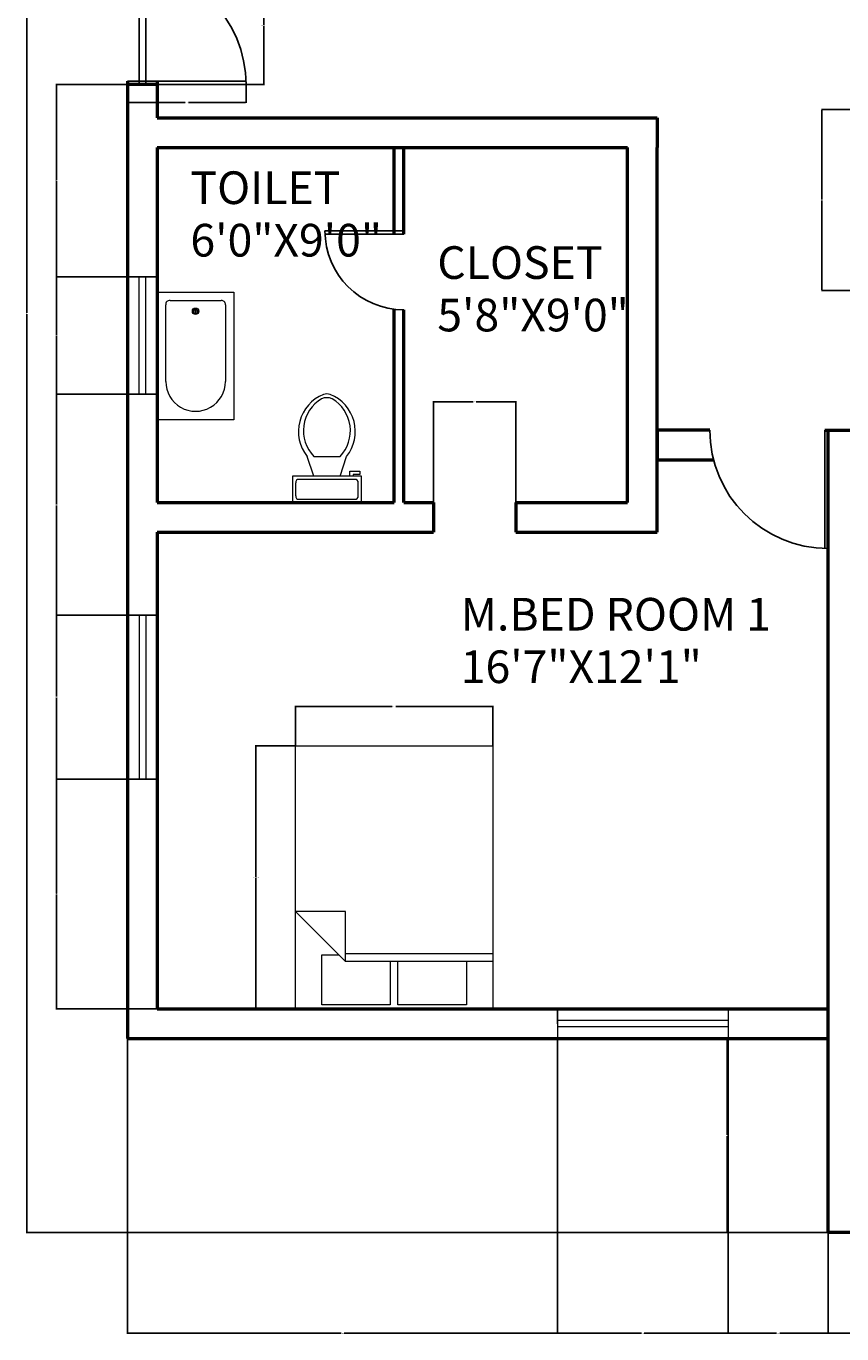
# Model space of a CAD drawing. Units: inches. Extents: x 614 to 1202, y 131 to 752.
# Tile 1 of 5: x 614 to 862, y 131 to 529. Entities that reach past the tile are written whole.
import ezdxf

# ---------------------------------------------------------------- set-up
doc = ezdxf.new("R2010")
doc.units = ezdxf.units.IN
doc.header["$MEASUREMENT"] = 0
for name, color, linetype, lineweight in [('A-ANNO-DIMS', 2, 'Continuous', 18), ('A-AREA-IDEN', 7, 'Continuous', 18), ('A-DOOR', 3, 'Continuous', 25), ('A-FLOR-FIXT', 9, 'Continuous', 18), ('A-FURN', 8, 'Continuous', 18), ('A-GLAZ', 4, 'Continuous', 18), ('A-WALL', 7, 'Continuous', 50)]:
    doc.layers.add(name, color=color, linetype=linetype, lineweight=lineweight)
doc.styles.get("Standard").update_dxf_attribs({"font": 'arial.ttf'})
doc.dimstyles.get("Standard").update_dxf_attribs({"dimtxt": 0.18, "dimasz": 0.18, "dimexe": 0.18, "dimexo": 0.0625, "dimgap": 0.09, "dimtad": 0, "dimtih": 1, "dimtoh": 1, "dimdec": 0, "dimzin": 0, "dimdsep": 46, "dimlunit": 3, "dimtxsty": 'Standard', "dimcen": 0.09, "dimadec": 0, "dimazin": 0, "dimtfac": 1, "dimtdec": 0, "dimtofl": 0, "dimtmove": 0, "dimatfit": 3, "dimfxl": 1, "dimtolj": 1, "dimtzin": 0, "dimarcsym": 0})

# ---------------------------------------------------------------- blocks, each defined once
blk = doc.blocks.new('Bed - Queen')
for p, q in [((0, -80.00003), (0, 0)), ((0, 0), (59.99999, 0)), ((59.99999, 0), (59.99999, -80.00003)), ((7.99999, -1.2), (28.79998, -1.2)), ((7.99999, -14.4), (7.99999, -1.2)), ((28.79998, -1.2), (28.79998, -14.4)), ((31.19999, -1.2), (51.99999, -1.2)), ((31.19999, -14.4), (31.19999, -1.2)), ((51.99999, -1.2), (51.99999, -16.4)), ((0, -14.4), (44.8, -14.4)), ((59.99999, -29.6), (44.8, -14.4)), ((44.8, -14.4), (44.8, -29.6)), ((44.8, -16.8), (0, -16.8)), ((51.99999, -16.4), (46.79936, -16.4)), ((44.8, -29.6), (59.99999, -29.6)), ((59.99999, -80.00003), (0, -80.00003))]:
    blk.add_line(p, q)
blk = doc.blocks.new('Toilet - top')
for p, q in [((9.5, -6), (9.5, -2)), ((-10, -8.5), (-8, -8.5)), ((-10, -9.5), (-10, -8.5)), ((-7, -9.5), (-10, -9.5)), ((-8, -8.5), (-8, -8)), ((-7, -8), (-7, -9.5)), ((-4, -8), (-6, -14)), ((4, -8), (6, -14)), ((4, -14), (-4, -14))]:
    blk.add_line(p, q)
blk.add_lwpolyline([(10.5, -8), (10.5, 0), (-10.5, 0), (-10.5, -8)], close=True)
for points in [[(-9.5, -2), (-9.5, -6)], [(8.5, -1), (-8.5, -1)], [(-8.5, -7), (8.5, -7)]]:
    blk.add_lwpolyline(points)
for centre, radius, start, end in [((-8.62, -1.88), 0.884, 81.8699, 188.1301), ((8.62, -1.88), 0.884, 351.8699, 98.1301), ((-8.62, -6.12), 0.884, 171.8699, 278.1301), ((8.62, -6.12), 0.884, 261.8699, 8.1301), ((3.52, -21.58), 12.17, 141.4691, 247.9714), ((4.2, -21.82), 11.33, 136.3677, 238.9468), ((-3.52, -21.58), 12.17, 292.0284, 38.5307), ((-4.2, -21.82), 11.33, 301.053, 43.6321), ((0, -27.88), 4, 245.7318, 294.2682), ((0, -29), 4, 254.8605, 285.1395)]:
    blk.add_arc(centre, radius, start, end)
blk = doc.blocks.new('Bath Tub - 26 x 60 in.')
for p, q in [((8, -18), (10, -18)), ((9, -17), (9, -19))]:
    blk.add_line(p, q)
blk.add_lwpolyline([(0, -36), (0, 0), (60, 0), (60, -36)], close=True)
for points in [[(4, -30), (4, -6)], [(6, -4), (42, -4)], [(42, -32), (6, -32)]]:
    blk.add_lwpolyline(points)
for radius in [1.5, 1]:
    blk.add_circle((9, -18), radius)
for centre, radius, start, end in [((5.75, -5.75), 1.77, 81.8699, 188.1301), ((42, -18), 14, 270, 90), ((5.75, -30.25), 1.77, 171.8699, 278.1301)]:
    blk.add_arc(centre, radius, start, end)
blk = doc.blocks.new('DOOR-SINGLE-36IN')
for p, q in [((0, 1), (36, 1)), ((0, 0), (36, 0))]:
    blk.add_line(p, q)
blk.add_arc((0, 0), 36, 0, 90)
blk = doc.blocks.new('DOOR-SINGLE-24IN')
for p, q in [((0, 0), (0, 24)), ((1, 0), (1, 24))]:
    blk.add_line(p, q)
blk.add_arc((0, 0), 24, 0, 90)
blk = doc.blocks.new('*D15')
at = {"layer": 'A-ANNO-DIMS', "color": 0, "lineweight": -2, "transparency": 16777216}
for p, q in [((681.06, 547.36), (686.57, 547.36)), ((686.39, 547.18), (686.39, 529.54)), ((686.39, 511.54), (686.39, 529.18)), ((681.06, 511.36), (686.57, 511.36))]:
    blk.add_line(p, q, dxfattribs=at)
at = {"layer": 'A-ANNO-DIMS', "color": 0, "transparency": 16777216}
for points in [[(686.36, 547.18), (686.42, 547.18), (686.39, 547.36)], [(686.36, 511.54), (686.42, 511.54), (686.39, 511.36)]]:
    blk.add_solid(points, dxfattribs=at)
at = {"layer": 'Defpoints', "color": 0, "transparency": 16777216}
for p in [(680.99, 547.36), (686.39, 547.36), (680.99, 511.36)]:
    blk.add_point(p, dxfattribs=at)
at = {"layer": 'A-ANNO-DIMS', "color": 0, "transparency": 16777216, "insert": (686.39, 529.36), "char_height": 0.18, "attachment_point": 5}
blk.add_mtext('\\A1;DOOR 36 TYP.', dxfattribs=at)
blk = doc.blocks.new('*D16')
at = {"layer": 'A-ANNO-DIMS', "color": 0, "lineweight": -2, "transparency": 16777216}
for p, q in [((644.99, 511.3), (644.99, 505.78)), ((680.99, 511.3), (680.99, 505.78)), ((645.17, 505.96), (662.47, 505.96)), ((680.81, 505.96), (663.52, 505.96))]:
    blk.add_line(p, q, dxfattribs=at)
at = {"layer": 'A-ANNO-DIMS', "color": 0, "transparency": 16777216}
for points in [[(645.17, 505.99), (645.17, 505.93), (644.99, 505.96)], [(680.81, 505.99), (680.81, 505.93), (680.99, 505.96)]]:
    blk.add_solid(points, dxfattribs=at)
at = {"layer": 'Defpoints', "color": 0, "transparency": 16777216}
for p in [(644.99, 511.36), (680.99, 511.36), (680.99, 505.96)]:
    blk.add_point(p, dxfattribs=at)
at = {"layer": 'A-ANNO-DIMS', "color": 0, "transparency": 16777216, "insert": (662.99, 505.96), "char_height": 0.18, "attachment_point": 5}
blk.add_mtext('\\A1;36 TYP.', dxfattribs=at)
blk = doc.blocks.new('*D23')
at = {"layer": 'A-ANNO-DIMS', "color": 0, "lineweight": -2, "transparency": 16777216}
for p, q in [((695.93, 310.26), (683.81, 310.26)), ((683.99, 310.08), (683.99, 270.45)), ((683.99, 230.44), (683.99, 270.08)), ((695.93, 230.26), (683.81, 230.26))]:
    blk.add_line(p, q, dxfattribs=at)
at = {"layer": 'A-ANNO-DIMS', "color": 0, "transparency": 16777216}
for points in [[(683.96, 310.08), (684.02, 310.08), (683.99, 310.26)], [(683.96, 230.44), (684.02, 230.44), (683.99, 230.26)]]:
    blk.add_solid(points, dxfattribs=at)
at = {"layer": 'Defpoints', "color": 0, "transparency": 16777216}
for p in [(695.99, 310.26), (683.99, 230.26), (695.99, 230.26)]:
    blk.add_point(p, dxfattribs=at)
at = {"layer": 'A-ANNO-DIMS', "color": 0, "transparency": 16777216, "insert": (683.99, 270.26), "char_height": 0.18, "attachment_point": 5}
blk.add_mtext('\\A1;QUEEN BED 80 TYP.', dxfattribs=at)
blk = doc.blocks.new('*D24')
at = {"layer": 'A-ANNO-DIMS', "color": 0, "lineweight": -2, "transparency": 16777216}
for p, q in [((695.99, 310.33), (695.99, 322.44)), ((696.17, 322.26), (725.47, 322.26)), ((755.81, 322.26), (726.52, 322.26)), ((755.99, 310.33), (755.99, 322.44))]:
    blk.add_line(p, q, dxfattribs=at)
at = {"layer": 'A-ANNO-DIMS', "color": 0, "transparency": 16777216}
for points in [[(696.17, 322.29), (696.17, 322.23), (695.99, 322.26)], [(755.81, 322.29), (755.81, 322.23), (755.99, 322.26)]]:
    blk.add_solid(points, dxfattribs=at)
at = {"layer": 'Defpoints', "color": 0, "transparency": 16777216}
for p in [(695.99, 322.26), (695.99, 310.26), (755.99, 310.26)]:
    blk.add_point(p, dxfattribs=at)
at = {"layer": 'A-ANNO-DIMS', "color": 0, "transparency": 16777216, "insert": (725.99, 322.26), "char_height": 0.18, "attachment_point": 5}
blk.add_mtext('\\A1;60 TYP.', dxfattribs=at)
blk = doc.blocks.new('*D34')
at = {"layer": 'A-ANNO-DIMS', "color": 0, "lineweight": -2, "transparency": 16777216}
for p, q in [((869.71, 503.76), (855.94, 503.76)), ((856.12, 503.58), (856.12, 476.44)), ((856.12, 448.94), (856.12, 476.08)), ((869.71, 448.76), (855.94, 448.76))]:
    blk.add_line(p, q, dxfattribs=at)
at = {"layer": 'A-ANNO-DIMS', "color": 0, "transparency": 16777216}
for points in [[(856.09, 503.58), (856.15, 503.58), (856.12, 503.76)], [(856.09, 448.94), (856.15, 448.94), (856.12, 448.76)]]:
    blk.add_solid(points, dxfattribs=at)
at = {"layer": 'Defpoints', "color": 0, "transparency": 16777216}
for p in [(856.12, 503.76), (869.77, 503.76), (869.77, 448.76)]:
    blk.add_point(p, dxfattribs=at)
at = {"layer": 'A-ANNO-DIMS', "color": 0, "transparency": 16777216, "insert": (856.12, 476.26), "char_height": 0.18, "attachment_point": 5}
blk.add_mtext('\\A1;55', dxfattribs=at)
blk = doc.blocks.new('*D36')
at = {"layer": 'A-ANNO-DIMS', "color": 0, "lineweight": -2, "transparency": 16777216}
for p, q in [((644.93, 721.26), (614.16, 721.26)), ((614.34, 721.08), (614.34, 441.95)), ((614.34, 162.44), (614.34, 441.58)), ((857.93, 162.26), (614.16, 162.26))]:
    blk.add_line(p, q, dxfattribs=at)
at = {"layer": 'A-ANNO-DIMS', "color": 0, "transparency": 16777216}
for points in [[(614.31, 721.08), (614.37, 721.08), (614.34, 721.26)], [(614.31, 162.44), (614.37, 162.44), (614.34, 162.26)]]:
    blk.add_solid(points, dxfattribs=at)
at = {"layer": 'Defpoints', "color": 0, "transparency": 16777216}
for p in [(614.34, 721.26), (644.99, 721.26), (857.99, 162.26)]:
    blk.add_point(p, dxfattribs=at)
at = {"layer": 'A-ANNO-DIMS', "color": 0, "transparency": 16777216, "insert": (614.34, 441.76), "char_height": 0.18, "attachment_point": 5}
blk.add_mtext('\\A1;559', dxfattribs=at)
blk = doc.blocks.new('*D47')
at = {"layer": 'A-ANNO-DIMS', "color": 0, "lineweight": -2, "transparency": 16777216}
for p, q in [((653.93, 511.36), (623.16, 511.36)), ((623.34, 511.18), (623.34, 482.33)), ((623.34, 453.11), (623.34, 481.96)), ((653.93, 452.93), (623.16, 452.93))]:
    blk.add_line(p, q, dxfattribs=at)
at = {"layer": 'A-ANNO-DIMS', "color": 0, "transparency": 16777216}
for points in [[(623.31, 511.18), (623.37, 511.18), (623.34, 511.36)], [(623.31, 453.11), (623.37, 453.11), (623.34, 452.93)]]:
    blk.add_solid(points, dxfattribs=at)
at = {"layer": 'Defpoints', "color": 0, "transparency": 16777216}
for p in [(623.34, 511.36), (653.99, 511.36), (653.99, 452.93)]:
    blk.add_point(p, dxfattribs=at)
at = {"layer": 'A-ANNO-DIMS', "color": 0, "transparency": 16777216, "insert": (623.34, 482.15), "char_height": 0.18, "attachment_point": 5}
blk.add_mtext('\\A1;58.42', dxfattribs=at)
blk = doc.blocks.new('*D48')
at = {"layer": 'A-ANNO-DIMS', "color": 0, "lineweight": -2, "transparency": 16777216}
for p, q in [((653.93, 452.93), (623.16, 452.93)), ((623.34, 452.75), (623.34, 435.26)), ((623.34, 417.4), (623.34, 434.9)), ((653.93, 417.22), (623.16, 417.22))]:
    blk.add_line(p, q, dxfattribs=at)
at = {"layer": 'A-ANNO-DIMS', "color": 0, "transparency": 16777216}
for points in [[(623.31, 452.75), (623.37, 452.75), (623.34, 452.93)], [(623.31, 417.4), (623.37, 417.4), (623.34, 417.22)]]:
    blk.add_solid(points, dxfattribs=at)
at = {"layer": 'Defpoints', "color": 0, "transparency": 16777216}
for p in [(623.34, 452.93), (653.99, 452.93), (653.99, 417.22)]:
    blk.add_point(p, dxfattribs=at)
at = {"layer": 'A-ANNO-DIMS', "color": 0, "transparency": 16777216, "insert": (623.34, 435.08), "char_height": 0.18, "attachment_point": 5}
blk.add_mtext('\\A1;35.71', dxfattribs=at)
blk = doc.blocks.new('*D49')
at = {"layer": 'A-ANNO-DIMS', "color": 0, "lineweight": -2, "transparency": 16777216}
for p, q in [((653.93, 417.22), (623.16, 417.22)), ((623.34, 417.04), (623.34, 383.77)), ((623.34, 350.13), (623.34, 383.4)), ((653.93, 349.95), (623.16, 349.95))]:
    blk.add_line(p, q, dxfattribs=at)
at = {"layer": 'A-ANNO-DIMS', "color": 0, "transparency": 16777216}
for points in [[(623.31, 417.04), (623.37, 417.04), (623.34, 417.22)], [(623.31, 350.13), (623.37, 350.13), (623.34, 349.95)]]:
    blk.add_solid(points, dxfattribs=at)
at = {"layer": 'Defpoints', "color": 0, "transparency": 16777216}
for p in [(623.34, 417.22), (653.99, 417.22), (653.99, 349.95)]:
    blk.add_point(p, dxfattribs=at)
at = {"layer": 'A-ANNO-DIMS', "color": 0, "transparency": 16777216, "insert": (623.34, 383.58), "char_height": 0.18, "attachment_point": 5}
blk.add_mtext('\\A1;67.28', dxfattribs=at)
blk = doc.blocks.new('*D50')
at = {"layer": 'A-ANNO-DIMS', "color": 0, "lineweight": -2, "transparency": 16777216}
for p, q in [((653.93, 349.95), (623.16, 349.95)), ((623.34, 349.77), (623.34, 325.24)), ((623.34, 300.35), (623.34, 324.87)), ((653.93, 300.17), (623.16, 300.17))]:
    blk.add_line(p, q, dxfattribs=at)
at = {"layer": 'A-ANNO-DIMS', "color": 0, "transparency": 16777216}
for points in [[(623.31, 349.77), (623.37, 349.77), (623.34, 349.95)], [(623.31, 300.35), (623.37, 300.35), (623.34, 300.17)]]:
    blk.add_solid(points, dxfattribs=at)
at = {"layer": 'Defpoints', "color": 0, "transparency": 16777216}
for p in [(623.34, 349.95), (653.99, 349.95), (653.99, 300.17)]:
    blk.add_point(p, dxfattribs=at)
at = {"layer": 'A-ANNO-DIMS', "color": 0, "transparency": 16777216, "insert": (623.34, 325.06), "char_height": 0.18, "attachment_point": 5}
blk.add_mtext('\\A1;49.78', dxfattribs=at)
blk = doc.blocks.new('*D51')
at = {"layer": 'A-ANNO-DIMS', "color": 0, "lineweight": -2, "transparency": 16777216}
for p, q in [((653.93, 300.17), (623.16, 300.17)), ((623.34, 299.99), (623.34, 265.4)), ((623.34, 230.44), (623.34, 265.03)), ((653.93, 230.26), (623.16, 230.26))]:
    blk.add_line(p, q, dxfattribs=at)
at = {"layer": 'A-ANNO-DIMS', "color": 0, "transparency": 16777216}
for points in [[(623.31, 299.99), (623.37, 299.99), (623.34, 300.17)], [(623.31, 230.44), (623.37, 230.44), (623.34, 230.26)]]:
    blk.add_solid(points, dxfattribs=at)
at = {"layer": 'Defpoints', "color": 0, "transparency": 16777216}
for p in [(623.34, 300.17), (653.99, 300.17), (653.99, 230.26)]:
    blk.add_point(p, dxfattribs=at)
at = {"layer": 'A-ANNO-DIMS', "color": 0, "transparency": 16777216, "insert": (623.34, 265.21), "char_height": 0.18, "attachment_point": 5}
blk.add_mtext('\\A1;69.9', dxfattribs=at)
blk = doc.blocks.new('*D61')
at = {"layer": 'A-ANNO-DIMS', "color": 0, "lineweight": -2, "transparency": 16777216}
for p, q in [((644.99, 221.2), (644.99, 131.43)), ((775.74, 221.2), (775.74, 131.43)), ((645.17, 131.61), (709.91, 131.61)), ((775.56, 131.61), (710.82, 131.61))]:
    blk.add_line(p, q, dxfattribs=at)
at = {"layer": 'A-ANNO-DIMS', "color": 0, "transparency": 16777216}
for points in [[(645.17, 131.64), (645.17, 131.58), (644.99, 131.61)], [(775.56, 131.64), (775.56, 131.58), (775.74, 131.61)]]:
    blk.add_solid(points, dxfattribs=at)
at = {"layer": 'Defpoints', "color": 0, "transparency": 16777216}
for p in [(644.99, 221.26), (775.74, 221.26), (775.74, 131.61)]:
    blk.add_point(p, dxfattribs=at)
at = {"layer": 'A-ANNO-DIMS', "color": 0, "transparency": 16777216, "insert": (710.37, 131.61), "char_height": 0.18, "attachment_point": 5}
blk.add_mtext('\\A1;130.75', dxfattribs=at)
blk = doc.blocks.new('*D62')
at = {"layer": 'A-ANNO-DIMS', "color": 0, "lineweight": -2, "transparency": 16777216}
for p, q in [((775.74, 221.2), (775.74, 131.43)), ((827.61, 221.2), (827.61, 131.43)), ((775.92, 131.61), (801.28, 131.61)), ((827.43, 131.61), (802.07, 131.61))]:
    blk.add_line(p, q, dxfattribs=at)
at = {"layer": 'A-ANNO-DIMS', "color": 0, "transparency": 16777216}
for points in [[(775.92, 131.64), (775.92, 131.58), (775.74, 131.61)], [(827.43, 131.64), (827.43, 131.58), (827.61, 131.61)]]:
    blk.add_solid(points, dxfattribs=at)
at = {"layer": 'Defpoints', "color": 0, "transparency": 16777216}
for p in [(775.74, 221.26), (827.61, 221.26), (827.61, 131.61)]:
    blk.add_point(p, dxfattribs=at)
at = {"layer": 'A-ANNO-DIMS', "color": 0, "transparency": 16777216, "insert": (801.68, 131.61), "char_height": 0.18, "attachment_point": 5}
blk.add_mtext('\\A1;51.86', dxfattribs=at)
blk = doc.blocks.new('*D63')
at = {"layer": 'A-ANNO-DIMS', "color": 0, "lineweight": -2, "transparency": 16777216}
for p, q in [((827.61, 221.2), (827.61, 131.43)), ((857.99, 162.2), (857.99, 131.43)), ((827.79, 131.61), (842.34, 131.61)), ((857.81, 131.61), (843.26, 131.61))]:
    blk.add_line(p, q, dxfattribs=at)
at = {"layer": 'A-ANNO-DIMS', "color": 0, "transparency": 16777216}
for points in [[(827.79, 131.64), (827.79, 131.58), (827.61, 131.61)], [(857.81, 131.64), (857.81, 131.58), (857.99, 131.61)]]:
    blk.add_solid(points, dxfattribs=at)
at = {"layer": 'Defpoints', "color": 0, "transparency": 16777216}
for p in [(827.61, 221.26), (857.99, 162.26), (857.99, 131.61)]:
    blk.add_point(p, dxfattribs=at)
at = {"layer": 'A-ANNO-DIMS', "color": 0, "transparency": 16777216, "insert": (842.8, 131.61), "char_height": 0.18, "attachment_point": 5}
blk.add_mtext('\\A1;30.386', dxfattribs=at)
blk = doc.blocks.new('*D64')
at = {"layer": 'A-ANNO-DIMS', "color": 0, "lineweight": -2, "transparency": 16777216}
for p, q in [((857.99, 162.2), (857.99, 131.43)), ((1016.99, 162.2), (1016.99, 131.43)), ((858.17, 131.61), (937.21, 131.61)), ((1016.81, 131.61), (937.77, 131.61))]:
    blk.add_line(p, q, dxfattribs=at)
at = {"layer": 'A-ANNO-DIMS', "color": 0, "transparency": 16777216}
for points in [[(858.17, 131.64), (858.17, 131.58), (857.99, 131.61)], [(1016.81, 131.64), (1016.81, 131.58), (1016.99, 131.61)]]:
    blk.add_solid(points, dxfattribs=at)
at = {"layer": 'Defpoints', "color": 0, "transparency": 16777216}
for p in [(857.99, 162.26), (1016.99, 162.26), (1016.99, 131.61)]:
    blk.add_point(p, dxfattribs=at)
at = {"layer": 'A-ANNO-DIMS', "color": 0, "transparency": 16777216, "insert": (937.49, 131.61), "char_height": 0.18, "attachment_point": 5}
blk.add_mtext('\\A1;159', dxfattribs=at)
blk = doc.blocks.new('*D68')
at = {"layer": 'A-ANNO-DIMS', "color": 0, "lineweight": -2, "transparency": 16777216}
for p, q in [((857.93, 221.26), (827.16, 221.26)), ((827.34, 221.08), (827.34, 191.95)), ((827.34, 162.44), (827.34, 191.58)), ((857.93, 162.26), (827.16, 162.26))]:
    blk.add_line(p, q, dxfattribs=at)
at = {"layer": 'A-ANNO-DIMS', "color": 0, "transparency": 16777216}
for points in [[(827.31, 221.08), (827.37, 221.08), (827.34, 221.26)], [(827.31, 162.44), (827.37, 162.44), (827.34, 162.26)]]:
    blk.add_solid(points, dxfattribs=at)
at = {"layer": 'Defpoints', "color": 0, "transparency": 16777216}
for p in [(827.34, 221.26), (857.99, 221.26), (857.99, 162.26)]:
    blk.add_point(p, dxfattribs=at)
at = {"layer": 'A-ANNO-DIMS', "color": 0, "transparency": 16777216, "insert": (827.34, 191.76), "char_height": 0.18, "attachment_point": 5}
blk.add_mtext('\\A1;59', dxfattribs=at)
blk = doc.blocks.new('*D79')
at = {"layer": 'A-ANNO-DIMS', "color": 0, "lineweight": -2, "transparency": 16777216}
for p, q in [((737.99, 384.33), (737.99, 415.09)), ((738.17, 414.91), (750.03, 414.91)), ((762.81, 414.91), (750.96, 414.91)), ((762.99, 384.33), (762.99, 415.09))]:
    blk.add_line(p, q, dxfattribs=at)
at = {"layer": 'A-ANNO-DIMS', "color": 0, "transparency": 16777216}
for points in [[(738.17, 414.94), (738.17, 414.88), (737.99, 414.91)], [(762.81, 414.94), (762.81, 414.88), (762.99, 414.91)]]:
    blk.add_solid(points, dxfattribs=at)
at = {"layer": 'Defpoints', "color": 0, "transparency": 16777216}
for p in [(762.99, 414.91), (737.99, 384.26), (762.99, 384.26)]:
    blk.add_point(p, dxfattribs=at)
at = {"layer": 'A-ANNO-DIMS', "color": 0, "transparency": 16777216, "insert": (750.49, 414.91), "char_height": 0.18, "attachment_point": 5}
blk.add_mtext('\\A1;25.006', dxfattribs=at)

msp = doc.modelspace()

# ---------------------------------------------------------------- linework, layer by layer
at = {"layer": 'A-DOOR'}
for p, q in [((648.4938, 511.3589), (648.4938, 547.1883)), ((650.4938, 511.3589), (650.4938, 546.9362)), ((644.9938, 511.3589), (644.9938, 512.3589)), ((728.9938, 466.8602), (728.9938, 465.8602))]:
    msp.add_line(p, q, dxfattribs=at)
at = {"layer": 'A-GLAZ'}
for p, q in [((653.9938, 452.934), (644.9938, 452.934)), ((648.4938, 417.2227), (648.4938, 452.934)), ((649.4938, 452.934), (653.9938, 452.934)), ((650.4938, 417.2227), (650.4938, 452.934)), ((653.9938, 417.2227), (644.9938, 417.2227)), ((653.9938, 349.9459), (644.9938, 349.9459)), ((648.4938, 349.9459), (648.4938, 300.1655)), ((650.4938, 349.9459), (650.4938, 300.1655)), ((653.9938, 300.1655), (644.9938, 300.1655)), ((649.4938, 300.1655), (653.9938, 300.1655)), ((775.7442, 225.7636), (775.7442, 230.2636)), ((775.7442, 230.2636), (775.7442, 221.2636)), ((827.6082, 226.7636), (775.7442, 226.7636)), ((827.6082, 230.2636), (827.6082, 221.2636)), ((827.6082, 224.7636), (775.7442, 224.7636))]:
    msp.add_line(p, q, dxfattribs=at)
at = {"layer": 'A-WALL'}
for p, q in [((644.9938, 512.3589), (644.9938, 221.2636)), ((653.9938, 511.3589), (644.9938, 511.3589)), ((653.9938, 512.3589), (653.9938, 501.2636)), ((653.9938, 501.2636), (797.9938, 501.2636)), ((797.9938, 501.2636), (805.9938, 501.2636)), ((805.9938, 501.2636), (805.9938, 492.2636)), ((644.9938, 492.2636), (644.9938, 384.2636)), ((653.9938, 492.2636), (796.9938, 492.2636)), ((653.9938, 492.2636), (653.9938, 384.2636)), ((725.9938, 465.8602), (725.9938, 492.2636)), ((728.9938, 465.8602), (728.9938, 492.2636)), ((796.9938, 384.2636), (796.9938, 492.2636)), ((805.9938, 375.2636), (805.9938, 492.2636)), ((725.9938, 384.2636), (725.9938, 443.0485)), ((728.9938, 384.2636), (728.9938, 442.8602)), ((821.9938, 406.2636), (805.9938, 406.2636)), ((805.9938, 406.2636), (805.9938, 397.2636)), ((856.9938, 406.2636), (866.9938, 406.2636)), ((857.9938, 255.2636), (857.9938, 406.2636)), ((805.9938, 397.2636), (823.1369, 397.2636)), ((653.9938, 384.2636), (725.9938, 384.2636)), ((728.9938, 384.2636), (737.9876, 384.2636)), ((737.9876, 384.2636), (737.9876, 375.2636)), ((762.9938, 384.2636), (762.9938, 375.2636)), ((762.9938, 384.2636), (796.9938, 384.2636)), ((644.9938, 375.2636), (644.9938, 230.2636)), ((653.9938, 375.2636), (737.9876, 375.2636)), ((653.9938, 375.2636), (653.9938, 230.2636)), ((728.9938, 375.2636), (737.9876, 375.2636)), ((762.9938, 375.2636), (796.9938, 375.2636)), ((762.9938, 375.2636), (805.9938, 375.2636)), ((857.9938, 162.2636), (857.9938, 255.2636)), ((653.9938, 230.2636), (857.9938, 230.2636)), ((644.9938, 221.2636), (857.9938, 221.2636)), ((1016.9938, 162.2636), (857.9938, 162.2636))]:
    msp.add_line(p, q, dxfattribs=at)

# ---------------------------------------------------------------- block references
at = {"layer": 'A-DOOR'}
msp.add_blockref('DOOR-SINGLE-36IN', (644.994, 511.359), dxfattribs=at)
at = {"layer": 'A-DOOR', "extrusion": (0, 0, -1), "zscale": -1}
for name, p, rotation in [('DOOR-SINGLE-24IN', (-728.9933, 466.8599), 270.0000000000002), ('DOOR-SINGLE-36IN', (-857.9936, 406.2633), 270.0000000000005)]:
    msp.add_blockref(name, p, dxfattribs=dict(at, rotation=rotation))
at = {"layer": 'A-FLOR-FIXT', "xscale": 0.6476301684216574, "yscale": 0.6476301684216574, "zscale": 0.6476301684216574, "rotation": 270}
msp.add_blockref('Bath Tub - 26 x 60 in.', (677.3084, 448.2637), dxfattribs=at)
at = {"layer": 'A-FLOR-FIXT', "rotation": 180}
msp.add_blockref('Toilet - top', (705.583, 384.2636), dxfattribs=at)
at = {"layer": 'A-FURN', "rotation": 180}
msp.add_blockref('Bed - Queen', (755.9938, 230.2636), dxfattribs=at)

# ---------------------------------------------------------------- texts
at = {"layer": 'A-AREA-IDEN'}
for s, p in [('TOILET', (664.0856, 475.024)), ('6\'0"X9\'0"', (664.0856, 459.0615)), ('CLOSET', (739.1558, 452.2615)), ('5\'8"X9\'0"', (739.1558, 436.299)), ('M.BED ROOM 1', (746.2872, 345.3105)), ('16\'7"X12\'1"', (746.2872, 329.348))]:
    msp.add_text(s, height=9.93672, dxfattribs=at).set_placement(p)

# ---------------------------------------------------------------- dimensions: what is measured, and where the dimension line sits
at = {"layer": 'A-ANNO-DIMS'}
for base, p1, p2, override, picture, middle in [((614.3438, 721.2636), (857.9938, 162.2636), (644.9938, 721.2636), {"dimdec": 0, "dimlfac": 1, "dimrnd": 0, "dimzin": 0, "dimdsep": 46, "dimlunit": 2}, '*D36', (614.3438, 441.7636)), ((623.3438, 511.3589), (653.9938, 452.934), (653.9938, 511.3589), {"dimdec": 2, "dimlfac": 1, "dimrnd": 0, "dimzin": 0, "dimdsep": 46, "dimlunit": 2}, '*D47', (623.3438, 482.1464)), ((856.1238, 503.7604), (869.7738, 448.7604), (869.7738, 503.7604), {"dimdec": 0, "dimlfac": 1, "dimrnd": 0, "dimzin": 0, "dimdsep": 46, "dimlunit": 2}, '*D34', (856.1238, 476.2604)), ((623.3438, 452.934), (653.9938, 417.2227), (653.9938, 452.934), {"dimdec": 2, "dimlfac": 1, "dimrnd": 0, "dimzin": 0, "dimdsep": 46, "dimlunit": 2}, '*D48', (623.3438, 435.0783)), ((623.3438, 417.2227), (653.9938, 349.9459), (653.9938, 417.2227), {"dimdec": 2, "dimlfac": 1, "dimrnd": 0, "dimzin": 0, "dimdsep": 46, "dimlunit": 2}, '*D49', (623.3438, 383.5843)), ((623.3438, 349.9459), (653.9938, 300.1655), (653.9938, 349.9459), {"dimdec": 2, "dimlfac": 1, "dimrnd": 0, "dimzin": 0, "dimdsep": 46, "dimlunit": 2}, '*D50', (623.3438, 325.0557)), ((623.3438, 300.1655), (653.9938, 230.2636), (653.9938, 300.1655), {"dimdec": 1, "dimlfac": 1, "dimrnd": 0, "dimzin": 0, "dimdsep": 46, "dimlunit": 2}, '*D51', (623.3438, 265.2145)), ((827.3438, 221.2636), (857.9938, 162.2636), (857.9938, 221.2636), {"dimdec": 0, "dimlfac": 1, "dimrnd": 0, "dimzin": 0, "dimdsep": 46, "dimlunit": 2}, '*D68', (827.3438, 191.7636))]:
    dim = msp.add_linear_dim(base=base, p1=p1, p2=p2, angle=90, dimstyle='Standard', override=override, dxfattribs=at)
    dim.commit()
    dim.dimension.update_dxf_attribs({"geometry": picture, "text_midpoint": middle})
for base, p1, p2, angle, text, picture, middle in [((686.3938, 547.3589), (680.9938, 511.3589), (680.9938, 547.3589), 90, 'DOOR <> TYP.', '*D15', (686.3938, 529.3589)), ((695.9938, 322.2636), (755.9938, 310.2636), (695.9938, 310.2636), 180, '<> TYP.', '*D24', (725.9938, 322.2636)), ((683.9938, 230.2636), (695.9938, 310.2636), (695.9938, 230.2636), 270, 'QUEEN BED <> TYP.', '*D23', (683.9938, 270.2636))]:
    dim = msp.add_linear_dim(base=base, p1=p1, p2=p2, angle=angle, text=text, dimstyle='Standard', override={"dimdec": 0, "dimlfac": 1, "dimrnd": 0, "dimzin": 0, "dimdsep": 46, "dimlunit": 2}, dxfattribs=at)
    dim.commit()
    dim.dimension.update_dxf_attribs({"geometry": picture, "text_midpoint": middle})
dim = msp.add_linear_dim(base=(680.9938, 505.9589), p1=(644.9938, 511.3589), p2=(680.9938, 511.3589), text='<> TYP.', dimstyle='Standard', override={"dimdec": 0, "dimlfac": 1, "dimrnd": 0, "dimzin": 0, "dimdsep": 46, "dimlunit": 2}, dxfattribs=at)
dim.commit()
dim.dimension.update_dxf_attribs({"geometry": '*D16', "text_midpoint": (662.9938, 505.9589)})
for base, p1, p2, override, picture, middle in [((762.9938, 414.9136), (737.9876, 384.2636), (762.9938, 384.2636), {"dimdec": 3, "dimlfac": 1, "dimrnd": 0, "dimzin": 0, "dimdsep": 46, "dimlunit": 2}, '*D79', (750.4907, 414.9136)), ((775.7442, 131.6136), (644.9938, 221.2636), (775.7442, 221.2636), {"dimdec": 2, "dimlfac": 1, "dimrnd": 0, "dimzin": 0, "dimdsep": 46, "dimlunit": 2}, '*D61', (710.369, 131.6136)), ((827.6082, 131.6136), (775.7442, 221.2636), (827.6082, 221.2636), {"dimdec": 2, "dimlfac": 1, "dimrnd": 0, "dimzin": 0, "dimdsep": 46, "dimlunit": 2}, '*D62', (801.6762, 131.6136)), ((857.9938, 131.6136), (827.6082, 221.2636), (857.9938, 162.2636), {"dimdec": 3, "dimlfac": 1, "dimrnd": 0, "dimzin": 0, "dimdsep": 46, "dimlunit": 2}, '*D63', (842.801, 131.6136)), ((1016.9938, 131.6136), (857.9938, 162.2636), (1016.9938, 162.2636), {"dimdec": 0, "dimlfac": 1, "dimrnd": 0, "dimzin": 0, "dimdsep": 46, "dimlunit": 2}, '*D64', (937.4938, 131.6136))]:
    dim = msp.add_linear_dim(base=base, p1=p1, p2=p2, dimstyle='Standard', override=override, dxfattribs=at)
    dim.commit()
    dim.dimension.update_dxf_attribs({"geometry": picture, "text_midpoint": middle})

doc.saveas('drawing.dxf')
